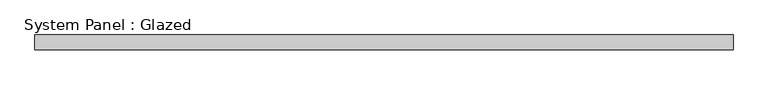
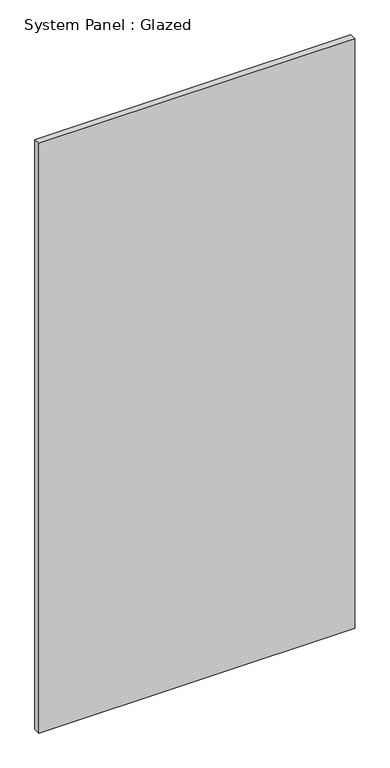
"""IFC4 building model written with IfcOpenShell, lengths in millimetres: plate geometry, System Panel : Glazed."""

from ifc_helpers import new_model, si_unit, origin, origin_with_axes, place, context, project, spatial, polyline, outline, extrude, source, transform, mapped, element, save


def system_panel_glazed_153bb9bb(model_context):
    return source(origin(), model_context, "Body", "SweptSolid", [
        extrude(outline(polyline([(593.725, -44.45), (-593.725, -44.45), (-593.725, -19.05), (593.725, -19.05), (593.725, -44.45)])), origin_with_axes(), (0.0, 0.0, 1.0), 2343.15),
    ])


if __name__ == "__main__":
    model = new_model("IFC4")
    model_context = context("Model", 3, world=origin())
    ifc_project = project(units=[si_unit("LENGTHUNIT", "METRE", prefix="MILLI")], contexts=[model_context])
    site = spatial("IfcSite", under=ifc_project)
    building = spatial("IfcBuilding", under=site)
    placement = place(None, origin())
    system_panel_glazed_shape = system_panel_glazed_153bb9bb(model_context)
    element("IfcPlate", 1, ObjectType="System Panel : Glazed", at=placement, inside=building, context=model_context, shape_type="MappedRepresentation", body=[
        mapped(system_panel_glazed_shape, transform((0.0, 0.0, 0.0), x_axis=(1.0, 0.0, 0.0), y_axis=(0.0, 1.0, 0.0), z_axis=(0.0, 0.0, 1.0))),
    ])
    save(model, "model.ifc")

# Revit data of these elements
# Type "System Panel : Glazed"
#   Construction Type Id = "GSP4R"
#   Analytic Construction = "1/8 in Pilkington single glazing"
#   Visual Light Transmittance = 0.9
#   Solar Heat Gain Coefficient = 0.86
#   Heat Transfer Coefficient (U) = 1.18115 BTU/(h·ft²·°F)
# Element 1 (IfcPlate, "System Panel : Glazed")
#   Materials on its faces: "Glass"
# Materials
#   "Glass": class "Glass", colour RGB 0 128 192, transparency 0.75, Description = "Soda Lime Glass", Cost = 0
